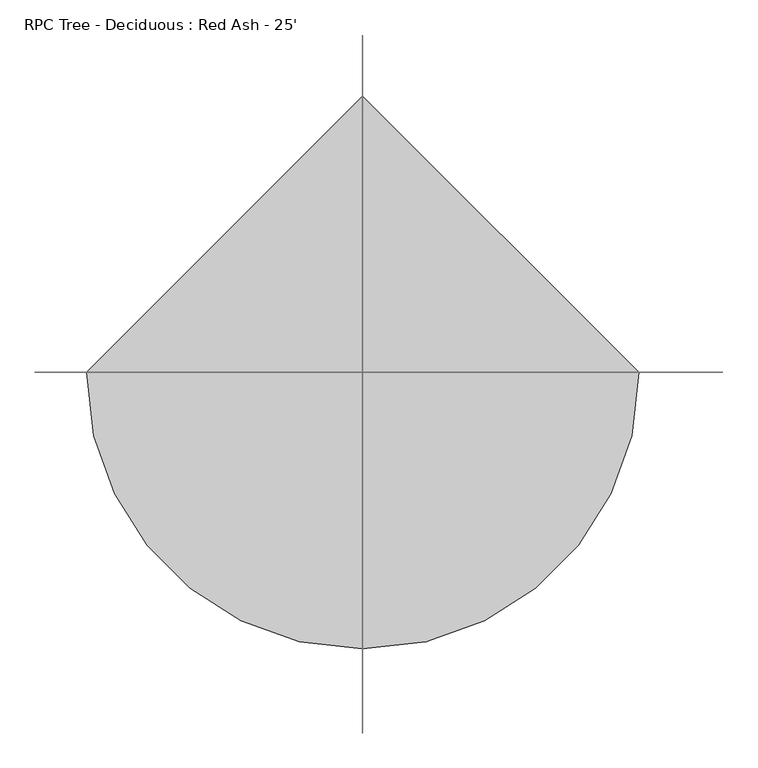
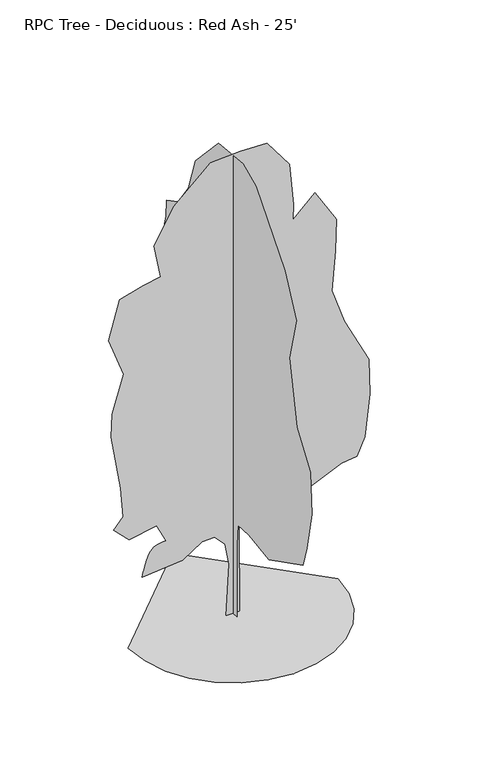
"""IFC4 building model written with IfcOpenShell, lengths in millimetres: geographic element geometry, RPC Tree - Deciduous : Red Ash - 25'."""

from ifc_helpers import new_model, si_unit, origin, place, context, project, spatial, triangles, source, transform, mapped, element, save


def rpc_tree_deciduous_red_ash_25_14781bec(model_context):
    return source(origin(), model_context, "Body", "Tessellation", [
        triangles([(-1644.9525009, 0.0, 6.19e-05), (-1601.4651844, -376.9143482, 6.19e-05), (-1477.6144592, -723.0498339, 6.19e-05), (-1283.3164352, -1028.4894024, 6.19e-05), (-1028.4894751, -1283.3165806, 6.19e-05), (-723.0496885, -1477.6140232, 6.19e-05), (-376.9141665, -1601.4651844, 6.19e-05), (7.19e-05, -1644.9525009, 6.19e-05), (376.9143846, -1601.4651844, 6.19e-05), (723.0499065, -1477.6143139, 6.19e-05), (1028.4894751, -1283.3164352, 6.19e-05), (1283.3168713, -1028.4894751, 6.19e-05), (1477.6141685, -723.0496159, 6.19e-05), (1601.4651844, -376.9140939, 6.19e-05), (1644.9525009, 0.0001438, 6.19e-05), (-0.0002157, 1644.9525009, 6.19e-05), (-1.07e-05, -102.8462569, 0.0), (2.5e-05, -101.2467179, 1194.554048), (3.23e-05, -129.8819613, 1537.8029366), (7e-07, -438.8253948, 1558.1655018), (-5.78e-05, -976.3912743, 1478.3068588), (-0.0001405, -1903.692667, 1948.6771305), (-0.0001413, -2011.2060173, 2298.095192), (-0.0001361, -2145.5975235, 2943.1744217), (-0.0001119, -2105.2803623, 3615.1319527), (-5.81e-05, -1740.3819958, 4141.0172951), (-5.5e-06, -1527.3986298, 5160.6350006), (-3.5e-06, -1715.5451397, 5886.3488434), (4.79e-05, -1406.4449661, 6531.4286545), (0.0001569, -626.9743755, 7458.7301926), (0.0001985, -273.2007115, 7618.1942963), (0.0002662, 394.4016166, 7552.8046829), (0.0003121, 1026.0418774, 6880.8468613), (0.0003149, 1214.190204, 6316.4022446), (0.0003323, 1496.411277, 5913.2274353), (0.0003598, 1805.5131947, 5751.9582092), (0.0003531, 1818.9521999, 5483.1746155), (0.0003523, 1899.587249, 5174.0742966), (0.0003275, 1765.1957428, 4811.2170845), (0.0003297, 1886.1480984, 4461.7991684), (0.0003279, 2007.1004539, 3977.9897461), (0.0003211, 1980.222298, 3843.5979492), (0.0002877, 1751.7567375, 3521.0580437), (0.0002729, 1737.3115437, 3077.5662186), (0.0002632, 1724.8782909, 2795.3439102), (0.0002542, 1738.3174416, 2445.9262848), (0.0002412, 1751.7568829, 1962.1167171), (0.0002172, 1563.6084835, 1814.2857697), (0.0001807, 1214.1907127, 1814.2857697), (0.0001827, 1375.4605202, 1317.0371967), (0.0001715, 1348.4951603, 1034.8845062), (0.0001516, 1103.0310734, 1227.8363914), (9.86e-05, 629.4626684, 1106.7075932), (9.8e-05, 551.7118183, 1357.0609165), (6.29e-05, 215.9127657, 1354.0025276), (5.03e-05, 130.8012366, 1228.3346169), (3.27e-05, 79.5493323, 818.2831198), (1.17e-05, 112.1660096, 1.28e-05), (-110.870867, 4.8e-06, 4.46e-05), (-66.7114758, -9.64e-05, 833.5016676), (-129.3072962, -0.000136, 1187.9435503), (-290.7878647, -0.00015, 1365.31768), (-483.6364677, -0.0001408, 1358.6964272), (-796.2678211, -0.000103, 1155.7673166), (-1427.9080456, -6.9e-05, 1102.0108595), (-1419.1706429, -7.35e-05, 1136.7646975), (-1409.8454853, -7.82e-05, 1172.6938271), (-1399.3449635, -8.32e-05, 1210.9736853), (-1387.0813225, -8.87e-05, 1252.7803631), (-1372.4668076, -9.49e-05, 1299.2876987), (-1354.9136639, -0.0001019, 1351.6733093), (-1333.8341366, -0.0001099, 1411.1111057), (-1307.2693336, -0.0001176, 1466.2392815), (-1274.3570984, -0.0001239, 1506.556588), (-1236.1555058, -0.0001289, 1534.5316246), (-1193.7220493, -0.0001329, 1552.6338627), (-1148.1152401, -0.0001362, 1563.3300121), (-1100.3923536, -0.000139, 1569.0895443), (-1051.6116829, -0.0001415, 1572.3809132), (-1199.4421944, -0.0001703, 1868.0423721), (-1629.4953049, -0.0001418, 1787.4073231), (-1871.3997253, -0.0001601, 2029.3124702), (-1723.5690685, -0.0001874, 2204.0214283), (-1763.886375, -0.0002433, 2687.8309959), (-1911.7170319, -0.0003442, 3588.2539421), (-1898.4807758, -0.0003892, 3961.1654823), (-1719.9175472, -0.0004688, 4563.3255295), (-1952.0346291, -0.0005347, 5200.9523071), (-1777.3253803, -0.000616, 5819.1535263), (-1414.4687496, -0.0006447, 5926.6667313), (-1138.413216, -0.0006626, 5975.3625961), (-1239.7599369, -0.0007228, 6517.9893585), (-930.6591093, -0.000802, 7068.9952606), (-352.7753057, -0.0008898, 7593.1219894), (117.5946844, -0.0009135, 7620.0), (534.2087442, -0.0009301, 7606.5601227), (883.626733, -0.0008893, 7136.1905777), (947.8720848, -0.00081, 6447.5180786), (938.6469212, -0.0007795, 6194.9695404), (1286.8011063, -0.0008333, 6517.9893585), (1622.7800171, -0.0007823, 5966.9840378), (1609.3410118, -0.0007196, 5446.5094116), (1549.4574577, -0.00064, 4800.6520317), (1743.7323727, -0.0005809, 4233.3331718), (2131.7640656, -0.0005067, 3469.1978371), (2144.1354034, -0.0004386, 2892.8094727), (2066.2719875, -0.0003531, 2204.021283), (1945.319632, -0.0003141, 1921.7989746), (1703.4147755, -0.0003004, 1894.9206734), (1233.0446491, -0.0002542, 1679.8941181), (816.4305439, -0.0002007, 1384.2328045), (257.4765441, -0.0002049, 1624.5688614), (93.0508701, -0.0001766, 1447.6347485), (104.1552431, -4.6e-06, 3.52e-05)], [[15, 16, 1], [14, 15, 1], [14, 1, 2], [13, 14, 2], [13, 2, 3], [13, 3, 4], [12, 13, 4], [11, 12, 4], [11, 4, 5], [11, 5, 6], [11, 6, 7], [11, 7, 8], [11, 8, 9], [11, 9, 10], [50, 51, 52], [57, 58, 17], [57, 17, 18], [56, 57, 18], [56, 18, 19], [55, 56, 19], [49, 50, 52], [52, 53, 54], [49, 52, 54], [35, 36, 37], [46, 47, 48], [46, 48, 49], [21, 22, 23], [20, 21, 23], [20, 23, 24], [20, 24, 25], [20, 25, 26], [19, 20, 26], [19, 26, 27], [45, 46, 49], [31, 32, 33], [30, 31, 33], [29, 30, 33], [29, 33, 34], [28, 29, 34], [27, 28, 34], [19, 27, 34], [19, 34, 35], [19, 35, 37], [19, 37, 38], [19, 38, 39], [19, 39, 40], [19, 40, 41], [19, 41, 42], [19, 42, 43], [19, 43, 44], [19, 44, 45], [19, 45, 49], [19, 49, 54], [55, 19, 54], [64, 65, 66], [64, 66, 67], [64, 67, 68], [99, 100, 101], [64, 68, 69], [64, 69, 70], [64, 70, 71], [114, 59, 60], [113, 114, 60], [113, 60, 61], [113, 61, 62], [64, 71, 72], [64, 72, 73], [64, 73, 74], [64, 74, 75], [64, 75, 76], [64, 76, 77], [64, 77, 78], [64, 78, 79], [63, 64, 79], [81, 82, 83], [80, 81, 83], [99, 101, 102], [107, 108, 109], [110, 111, 112], [88, 89, 90], [87, 88, 90], [87, 90, 91], [80, 83, 84], [95, 96, 97], [95, 97, 98], [94, 95, 98], [93, 94, 98], [92, 93, 98], [91, 92, 98], [91, 98, 99], [87, 91, 99], [87, 99, 102], [87, 102, 103], [87, 103, 104], [86, 87, 104], [85, 86, 104], [84, 85, 104], [80, 84, 104], [80, 104, 105], [80, 105, 106], [80, 106, 107], [80, 107, 109], [80, 109, 110], [80, 110, 112], [79, 80, 112], [63, 79, 112], [62, 63, 112], [113, 62, 112]], closed=False),
    ])


if __name__ == "__main__":
    model = new_model("IFC4")
    model_context = context("Model", 3, world=origin())
    ifc_project = project(units=[si_unit("LENGTHUNIT", "METRE", prefix="MILLI")], contexts=[model_context])
    site = spatial("IfcSite", under=ifc_project)
    building = spatial("IfcBuilding", under=site)
    placement = place(None, origin())
    rpc_tree_deciduous_red_ash_25_shape = rpc_tree_deciduous_red_ash_25_14781bec(model_context)
    element("IfcGeographicElement", 1, ObjectType="RPC Tree - Deciduous : Red Ash - 25'", at=placement, inside=building, context=model_context, shape_type="MappedRepresentation", body=[
        mapped(rpc_tree_deciduous_red_ash_25_shape, transform((0.0, 0.0, 0.0), x_axis=(1.0, 0.0, 0.0), y_axis=(0.0, 1.0, 0.0), z_axis=(0.0, 0.0, 1.0))),
    ])
    save(model, "model.ifc")

# Revit data of these elements
# Type "RPC Tree - Deciduous : Red Ash - 25'"
#   built-in parameter 1005198 = "{2, 15},{22, RPC-8-G3GR-497X-PHW5-6},{1, 0},{1, 0},{2, 37},{1, 8},{5, Color},{1, 0},{1, 0},{3, 0.8},{3, 0.8},{3, 0.8},{1, 8},{7, BBoxMin},{1, 0},{1, 0},{1, 0},{1, 0},{1, 0},{1, 8},{7, BBoxMax},{1, 0},{1, 0},{1, 0},{1, 0},{1, 0},{2, 11},{9, RPCTypeId},{1, 0},{1, 0},{22, RPC-8-G3GR-497X-PHW5-6},{1, 6},{14, RPCPlantHeight},{1, 0},{1, 0},{2, 25},{2, 11},{7, keyword},{1, 0},{1, 0},{78, :Geometry:RPC:Red Ash:red ash:frainus pennsylvanica:frene rouge:deciduous:tree},{2, 11},{8, category},{1, 0},{1, 0},{16, :Trees [General]},{2, 11},{12, LocalizedUID},{1, 0},{1, 0},{7, Red Ash},{2, 14},{6, Height},{1, 0},{1, 0},{2, 25},{1, 2},{16, Cast Reflections},{1, 0},{1, 0},{1, 0},{1, 2},{6, Jitter},{1, 0},{1, 0},{1, 1},{1, 2},{9, Billboard},{1, 0},{1, 0},{1, 0},{1, 2},{12, Cast Shadows},{1, 0},{1, 0},{1, 1},{1, 2},{20, Apply Filter Effects},{1, 0},{1, 0},{1, 0},{2, 11},{28, Apply Filter Effects-Text-FC},{1, 0},{1, 0},{4, None},{2, 11},{20, AdvancedUIDefinition},{1, 0},{1, 0},{0, },{2, 11},{10, AssetLibID},{1, 0},{1, 0},{36, 4D3F6E72-3F99-4203-98E9-AF80B3C7A7A4},{2, 11},{10, BaseSchema},{1, 0},{1, 0},{9, RPCSchema},{2, 11},{12, ExchangeGUID},{1, 0},{1, 0},{0, },{1, 2},{6, Hidden},{1, 0},{1, 0},{1, 0},{1, 4},{11, RPCCategory},{1, 0},{1, 0},{1, 0},{2, 11},{8, RPCImage},{1, 0},{1, 0},{0, },{1, 4},{13, SchemaVersion},{1, 0},{1, 0},{1, 4},{2, 11},{12, UIDefinition},{1, 0},{1, 0},{0, },{2, 11},{6, UIName},{1, 0},{1, 0},{22, RPC-8-G3GR-497X-PHW5-6},{2, 11},{11, VersionGUID},{1, 0},{1, 0},{9, RPCSchema},{2, 11},{9, assettype},{1, 0},{1, 0},{11, RPCGeometry},{2, 11},{11, description},{1, 0},{1, 0},{0, },{2, 11},{9, localname},{1, 0},{1, 0},{3, RPC},{2, 11},{9, localtype},{1, 0},{1, 0},{3, RPC},{1, 4},{8, revision},{1, 0},{1, 0},{1, 1},{2, 11},{9, thumbnail},{1, 0},{1, 0},{0, },{1, 4},{7, version},{1, 0},{1, 0},{1, 1},{1, 2},{20, RPC_Cast Reflections},{1, 0},{1, 0},{1, 1},{1, 2},{10, RPC_Jitter},{1, 0},{1, 0},{1, 1},{1, 2},{13, RPC_Billboard},{1, 0},{1, 0},{1, 0},{1, 2},{16, RPC_Cast Shadows},{1, 0},{1, 0},{1, 1},{21, assetlibrary_base.fbx},{1, 5},"
#   built-in parameter 1005195 = "RPC-8-G3GR-497X-PHW5-6"
#   Type Comments = "Red Maple"
#   Assembly Code = "G2050500"
#   Height = 25' - 0"
#   Default Elevation = 0
